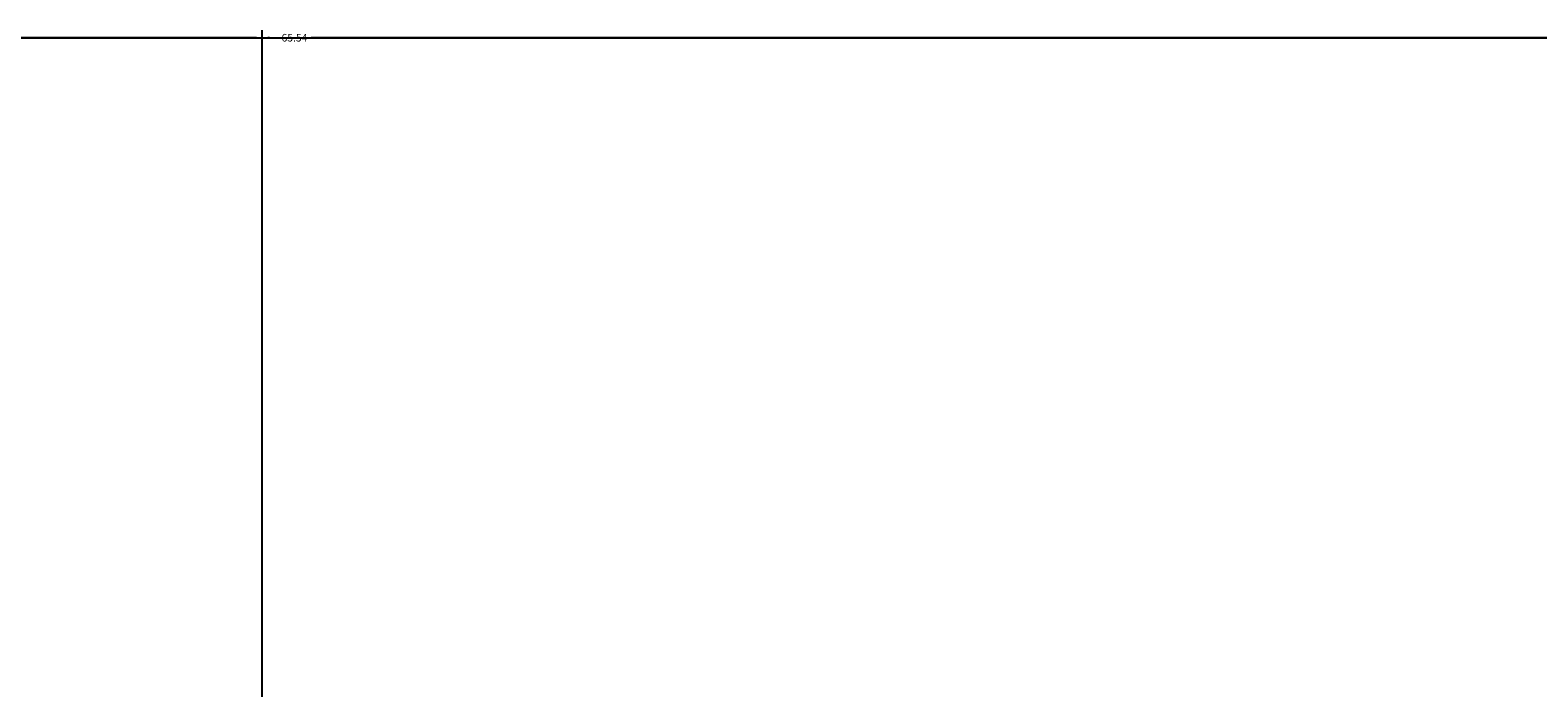
# Model space of a CAD drawing. Units: feet. Extents: x 2695 to 2912, y 795 to 1139.
# Tile 74 of 83: x 2805 to 2840, y 1123 to 1139. Entities that reach past the tile are written whole.
import ezdxf

# ---------------------------------------------------------------- set-up
doc = ezdxf.new("R2010")
doc.units = ezdxf.units.FT
doc.layers.add('A-ANNO-DIMS', color=2, linetype='Continuous', lineweight=18)
doc.styles.get("Standard").update_dxf_attribs({"font": 'arial.ttf'})
doc.dimstyles.get("Standard").update_dxf_attribs({"dimtxt": 0.18, "dimasz": 0.18, "dimexe": 0.18, "dimexo": 0.0625, "dimgap": 0.09, "dimtad": 0, "dimtih": 1, "dimtoh": 1, "dimdec": 1, "dimzin": 0, "dimdsep": 46, "dimlunit": 3, "dimtxsty": 'Standard', "dimcen": 0.09, "dimadec": 0, "dimazin": 0, "dimtfac": 1, "dimtdec": 1, "dimtofl": 0, "dimtmove": 0, "dimatfit": 3, "dimfxl": 1, "dimtolj": 1, "dimtzin": 0, "dimarcsym": 0})

# ---------------------------------------------------------------- blocks, each defined once
blk = doc.blocks.new('*D10')
at = {"layer": 'A-ANNO-DIMS', "color": 0, "lineweight": -2, "transparency": 16777216}
for p, q in [((2778.034, 1020.886), (2778.034, 1138.886)), ((2778.214, 1138.706), (2810.411, 1138.706)), ((2843.395, 1138.706), (2811.198, 1138.706)), ((2843.575, 1020.886), (2843.575, 1138.886))]:
    blk.add_line(p, q, dxfattribs=at)
at = {"layer": 'A-ANNO-DIMS', "color": 0, "transparency": 16777216}
for points in [[(2778.214, 1138.736), (2778.214, 1138.676), (2778.034, 1138.706)], [(2843.395, 1138.736), (2843.395, 1138.676), (2843.575, 1138.706)]]:
    blk.add_solid(points, dxfattribs=at)
at = {"layer": 'Defpoints', "color": 0, "transparency": 16777216}
for p in [(2843.575, 1138.706), (2778.034, 1020.824), (2843.575, 1020.824)]:
    blk.add_point(p, dxfattribs=at)
at = {"layer": 'A-ANNO-DIMS', "color": 0, "transparency": 16777216, "insert": (2810.805, 1138.706), "char_height": 0.18, "attachment_point": 5}
blk.add_mtext('\\A1;65.54', dxfattribs=at)
blk = doc.blocks.new('*D49')
at = {"layer": 'A-ANNO-DIMS', "color": 0, "lineweight": -2, "transparency": 16777216}
for p, q in [((2772.522, 972.03), (2772.522, 1138.886)), ((2772.702, 1138.706), (2790.888, 1138.706)), ((2809.861, 1138.706), (2791.674, 1138.706)), ((2810.041, 972.03), (2810.041, 1138.886))]:
    blk.add_line(p, q, dxfattribs=at)
at = {"layer": 'A-ANNO-DIMS', "color": 0, "transparency": 16777216}
for points in [[(2772.702, 1138.736), (2772.702, 1138.676), (2772.522, 1138.706)], [(2809.861, 1138.736), (2809.861, 1138.676), (2810.041, 1138.706)]]:
    blk.add_solid(points, dxfattribs=at)
at = {"layer": 'Defpoints', "color": 0, "transparency": 16777216}
for p in [(2810.041, 1138.706), (2772.522, 971.967), (2810.041, 971.967)]:
    blk.add_point(p, dxfattribs=at)
at = {"layer": 'A-ANNO-DIMS', "color": 0, "transparency": 16777216, "insert": (2791.281, 1138.706), "char_height": 0.18, "attachment_point": 5}
blk.add_mtext('\\A1;37.52', dxfattribs=at)
blk = doc.blocks.new('*D50')
at = {"layer": 'A-ANNO-DIMS', "color": 0, "lineweight": -2, "transparency": 16777216}
for p, q in [((2810.041, 972.03), (2810.041, 1138.886)), ((2810.221, 1138.706), (2848.721, 1138.706)), ((2888.008, 1138.706), (2849.508, 1138.706)), ((2888.188, 972.03), (2888.188, 1138.886))]:
    blk.add_line(p, q, dxfattribs=at)
at = {"layer": 'A-ANNO-DIMS', "color": 0, "transparency": 16777216}
for points in [[(2810.221, 1138.736), (2810.221, 1138.676), (2810.041, 1138.706)], [(2888.008, 1138.736), (2888.008, 1138.676), (2888.188, 1138.706)]]:
    blk.add_solid(points, dxfattribs=at)
at = {"layer": 'Defpoints', "color": 0, "transparency": 16777216}
for p in [(2888.188, 1138.706), (2810.041, 971.967), (2888.188, 971.967)]:
    blk.add_point(p, dxfattribs=at)
at = {"layer": 'A-ANNO-DIMS', "color": 0, "transparency": 16777216, "insert": (2849.114, 1138.706), "char_height": 0.18, "attachment_point": 5}
blk.add_mtext('\\A1;78.15', dxfattribs=at)

msp = doc.modelspace()

# ---------------------------------------------------------------- dimensions: what is measured, and where the dimension line sits
at = {"layer": 'A-ANNO-DIMS'}
for base, p1, p2, picture, middle in [((2810.0407, 1138.7056), (2772.5216, 971.9673), (2810.0407, 971.9673), '*D49', (2791.2811, 1138.7056)), ((2843.575, 1138.7056), (2778.0341, 1020.8235), (2843.575, 1020.8235), '*D10', (2810.8045, 1138.7056)), ((2888.1882, 1138.7056), (2810.0407, 971.9673), (2888.1882, 971.9673), '*D50', (2849.1144, 1138.7056))]:
    dim = msp.add_linear_dim(base=base, p1=p1, p2=p2, dimstyle='Standard', override={"dimdec": 2, "dimlfac": 1, "dimrnd": 0, "dimzin": 0, "dimdsep": 46, "dimlunit": 2}, dxfattribs=at)
    dim.commit()
    dim.dimension.update_dxf_attribs({"geometry": picture, "text_midpoint": middle})

doc.saveas('drawing.dxf')
